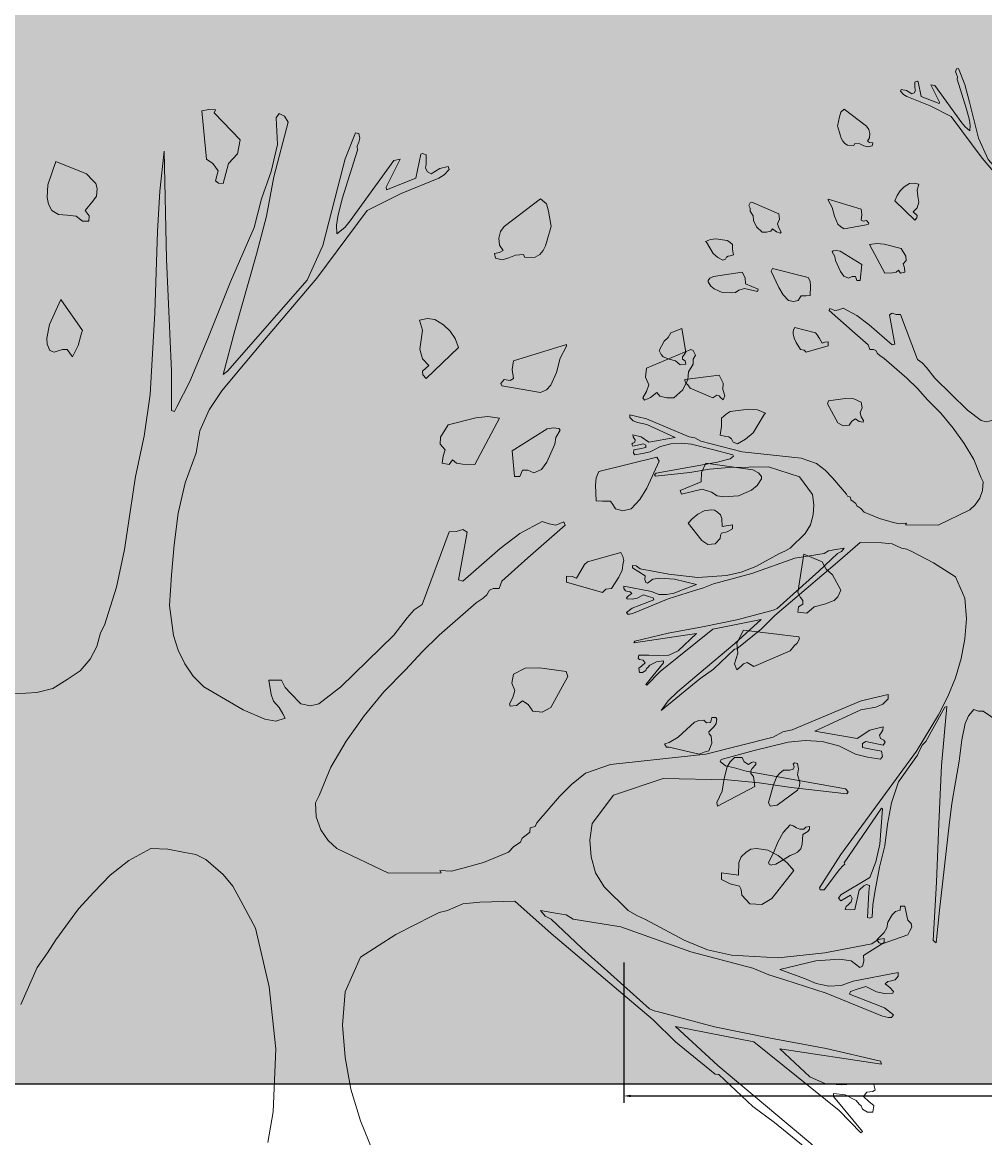
# Model space of a CAD drawing. Units: inches. Extents: x 84 to 1044, y -280 to 906.
# Tile 18 of 105: x 659 to 684, y -114 to -86. Entities that reach past the tile are written whole.
import ezdxf

# ---------------------------------------------------------------- set-up
doc = ezdxf.new("R2010")
doc.units = ezdxf.units.IN
for name, color, linetype, lineweight in [('A-ANNO-DIMS', 2, 'Continuous', 18), ('C-PROP', 7, 'Continuous', 25), ('L-PLNT', 114, 'Continuous', 15)]:
    doc.layers.add(name, color=color, linetype=linetype, lineweight=lineweight)
doc.layers.add('L-PLNT-PATT', color=9, linetype='Continuous', lineweight=9, true_color=0xafd9aa)
doc.styles.get("Standard").update_dxf_attribs({"font": 'arial.ttf'})
doc.dimstyles.get("Standard").update_dxf_attribs({"dimtxt": 0.18, "dimasz": 0.18, "dimexe": 0.18, "dimexo": 0.0625, "dimgap": 0.09, "dimtad": 0, "dimtih": 1, "dimtoh": 1, "dimdec": 4, "dimzin": 0, "dimdsep": 46, "dimtxsty": 'Standard', "dimcen": 0.09, "dimadec": 0, "dimazin": 0, "dimtfac": 1, "dimtdec": 4, "dimtofl": 0, "dimtmove": 0, "dimatfit": 3, "dimfxl": 1, "dimtolj": 1, "dimtzin": 0, "dimarcsym": 0})

# ---------------------------------------------------------------- blocks, each defined once
blk = doc.blocks.new('A$C37E508DF')
for p, q in [((0.6329, 1.5111), (0.6367, 1.5175)), ((0.6367, 1.5175), (0.6423, 1.5201)), ((0.6423, 1.5201), (0.6453, 1.5158)), ((0.6826, 1.493), (0.7096, 1.5209)), ((0.7083, 1.5239), (0.7152, 1.5244)), ((0.7096, 1.5209), (0.7083, 1.5239)), ((0.7152, 1.5244), (0.7225, 1.5231)), ((0.7225, 1.5231), (0.7174, 1.4729)), ((0.6475, 1.4545), (0.6329, 1.5111)), ((0.6453, 1.5158), (0.644, 1.4879)), ((0.5583, 1.4948), (0.5596, 1.4995)), ((0.5596, 1.4905), (0.5583, 1.4948)), ((0.5596, 1.4995), (0.563, 1.5003)), ((0.563, 1.5003), (0.5737, 1.4733)), ((0.6852, 1.4785), (0.6826, 1.493)), ((0.5613, 1.4862), (0.5596, 1.4905)), ((0.5608, 1.4823), (0.5613, 1.4862)), ((0.5767, 1.4317), (0.5608, 1.4823)), ((0.644, 1.4879), (0.6505, 1.46)), ((0.4897, 1.4772), (0.4935, 1.4789)), ((0.4897, 1.4678), (0.4897, 1.4772)), ((0.4935, 1.4789), (0.4952, 1.478)), ((0.4952, 1.478), (0.5004, 1.4532)), ((0.5313, 1.4437), (0.5167, 1.4729)), ((0.5167, 1.4729), (0.5231, 1.4716)), ((0.5231, 1.4716), (0.5686, 1.409)), ((0.5737, 1.4733), (0.5814, 1.4437)), ((0.6946, 1.4682), (0.6852, 1.4785)), ((0.7174, 1.4729), (0.7109, 1.4682)), ((0.7589, 1.3691), (0.7615, 1.481)), ((0.7615, 1.481), (0.7658, 1.4395)), ((0.8421, 1.4575), (0.8739, 1.4703)), ((0.8739, 1.4703), (0.882, 1.4463)), ((0.4657, 1.4622), (0.4669, 1.4652)), ((0.4708, 1.4566), (0.4657, 1.4622)), ((0.4669, 1.4652), (0.4755, 1.463)), ((0.4755, 1.463), (0.4845, 1.4575)), ((0.4845, 1.4575), (0.4884, 1.4596)), ((0.4884, 1.4596), (0.4905, 1.4635)), ((0.4905, 1.4635), (0.4897, 1.4678)), ((0.6505, 1.46), (0.6603, 1.4317)), ((0.6976, 1.4579), (0.6946, 1.4682)), ((0.7109, 1.4682), (0.7053, 1.4609)), ((0.7053, 1.4609), (0.7083, 1.4502)), ((0.4764, 1.4532), (0.4708, 1.4566)), ((0.5154, 1.4373), (0.4764, 1.4532)), ((0.5004, 1.4532), (0.5308, 1.4412)), ((0.6552, 1.4137), (0.6475, 1.4545)), ((0.7002, 1.4476), (0.6976, 1.4579)), ((0.7049, 1.448), (0.7002, 1.4476)), ((0.7083, 1.4502), (0.7049, 1.448)), ((0.831, 1.4424), (0.8323, 1.4476)), ((0.8323, 1.4476), (0.8357, 1.451)), ((0.8357, 1.451), (0.8421, 1.4575)), ((0.551, 1.4197), (0.5154, 1.4373)), ((0.5308, 1.4412), (0.5313, 1.4437)), ((0.5814, 1.4437), (0.5969, 1.3833)), ((0.7658, 1.4395), (0.7684, 1.3979)), ((0.8318, 1.4343), (0.831, 1.4424)), ((0.882, 1.4463), (0.8829, 1.433)), ((0.3628, 1.4189), (0.3649, 1.4266)), ((0.3649, 1.4266), (0.3709, 1.4317)), ((0.3709, 1.4317), (0.4086, 1.403)), ((0.5814, 1.4133), (0.5767, 1.4317)), ((0.6603, 1.4317), (0.668, 1.4021)), ((0.8353, 1.4292), (0.8318, 1.4343)), ((0.8434, 1.4197), (0.8353, 1.4292)), ((0.8816, 1.4262), (0.8781, 1.4197)), ((0.8829, 1.433), (0.8816, 1.4262)), ((0.3598, 1.403), (0.3628, 1.4189)), ((0.6029, 1.3494), (0.551, 1.4197)), ((0.5827, 1.4043), (0.5814, 1.4133)), ((0.6655, 1.3743), (0.6552, 1.4137)), ((0.8391, 1.4141), (0.8434, 1.4197)), ((0.8395, 1.4086), (0.8391, 1.4141)), ((0.8528, 1.4137), (0.846, 1.4086)), ((0.8619, 1.4146), (0.8528, 1.4137)), ((0.8709, 1.4154), (0.8619, 1.4146)), ((0.8781, 1.4197), (0.8709, 1.4154)), ((0.3602, 1.4021), (0.3598, 1.403)), ((0.364, 1.3888), (0.3602, 1.4021)), ((0.4086, 1.403), (0.4125, 1.3979)), ((0.5686, 1.409), (0.5741, 1.4021)), ((0.5741, 1.4021), (0.5823, 1.3953)), ((0.5823, 1.3953), (0.5827, 1.4043)), ((0.668, 1.4021), (0.6925, 1.3455)), ((0.846, 1.4086), (0.8395, 1.4086)), ((0.3657, 1.3828), (0.364, 1.3888)), ((0.4125, 1.3979), (0.4142, 1.391)), ((0.4142, 1.391), (0.4134, 1.3837)), ((0.7684, 1.3979), (0.771, 1.3134)), ((0.3683, 1.3781), (0.3657, 1.3828)), ((0.3718, 1.3738), (0.3683, 1.3781)), ((0.4134, 1.3837), (0.4099, 1.3781)), ((0.4099, 1.3781), (0.4134, 1.376)), ((0.5969, 1.3833), (0.6132, 1.3472)), ((0.3765, 1.3713), (0.3718, 1.3738)), ((0.3872, 1.3708), (0.3765, 1.3713)), ((0.3885, 1.3738), (0.3872, 1.3708)), ((0.3971, 1.3734), (0.3885, 1.3738)), ((0.4039, 1.3704), (0.3971, 1.3734)), ((0.4108, 1.3683), (0.4039, 1.3704)), ((0.4176, 1.37), (0.4108, 1.3683)), ((0.4134, 1.376), (0.4189, 1.3751)), ((0.4189, 1.3751), (0.4176, 1.37)), ((0.6882, 1.2949), (0.6655, 1.3743)), ((0.7538, 1.2529), (0.7589, 1.3691)), ((0.6595, 1.2829), (0.6029, 1.3494)), ((0.6132, 1.3472), (0.6959, 1.2529)), ((0.6925, 1.3455), (0.7161, 1.2868)), ((0.846, 1.2949), (0.8687, 1.3271)), ((0.8687, 1.3271), (0.8803, 1.3014)), ((0.771, 1.3134), (0.7761, 1.2285)), ((0.4648, 1.2945), (0.4717, 1.3009)), ((0.4717, 1.3009), (0.4807, 1.3065)), ((0.4807, 1.3065), (0.4884, 1.3074)), ((0.4884, 1.3074), (0.4965, 1.3057)), ((0.4965, 1.3057), (0.4935, 1.2954)), ((0.8803, 1.3014), (0.8833, 1.2872)), ((0.4562, 1.2774), (0.4597, 1.2868)), ((0.4597, 1.2868), (0.4648, 1.2945)), ((0.4935, 1.2954), (0.4948, 1.2855)), ((0.4948, 1.2855), (0.4961, 1.2756)), ((0.7002, 1.2495), (0.6882, 1.2949)), ((0.7161, 1.2868), (0.7349, 1.2422)), ((0.8473, 1.2924), (0.846, 1.2949)), ((0.8507, 1.2795), (0.8473, 1.2924)), ((0.8833, 1.2872), (0.8829, 1.2808)), ((0.2101, 1.2696), (0.2127, 1.2744)), ((0.2127, 1.2744), (0.2152, 1.2752)), ((0.2152, 1.2752), (0.2611, 1.2559)), ((0.3439, 1.2804), (0.3992, 1.2636)), ((0.3439, 1.2787), (0.3439, 1.2804)), ((0.3507, 1.2662), (0.3439, 1.2787)), ((0.4897, 1.2452), (0.4562, 1.2774)), ((0.4961, 1.2756), (0.4935, 1.2658)), ((0.6865, 1.2508), (0.6595, 1.2829)), ((0.8567, 1.2679), (0.8507, 1.2795)), ((0.8619, 1.2752), (0.8567, 1.2679)), ((0.867, 1.2752), (0.8619, 1.2752)), ((0.8713, 1.2739), (0.867, 1.2752)), ((0.8756, 1.2726), (0.8713, 1.2739)), ((0.8799, 1.2744), (0.8756, 1.2726)), ((0.8829, 1.2808), (0.8799, 1.2744)), ((0.2127, 1.2654), (0.2101, 1.2696)), ((0.2127, 1.2602), (0.2127, 1.2654)), ((0.3546, 1.2516), (0.3507, 1.2662)), ((0.3992, 1.2636), (0.4005, 1.2546)), ((0.4935, 1.2658), (0.4867, 1.2589)), ((0.2174, 1.2521), (0.2127, 1.2602)), ((0.2182, 1.2443), (0.2174, 1.2521)), ((0.2611, 1.2559), (0.262, 1.2465)), ((0.3602, 1.2383), (0.3546, 1.2516)), ((0.4005, 1.2546), (0.3992, 1.2452)), ((0.4867, 1.2589), (0.4935, 1.2529)), ((0.4935, 1.2529), (0.4931, 1.2491)), ((0.7015, 1.2323), (0.6865, 1.2508)), ((0.6959, 1.2529), (0.7002, 1.2495)), ((0.7538, 1.2122), (0.7538, 1.2529)), ((0.2234, 1.2336), (0.2182, 1.2443)), ((0.262, 1.2465), (0.2586, 1.2388)), ((0.2586, 1.2388), (0.2611, 1.2319)), ((0.3992, 1.2452), (0.4026, 1.2431)), ((0.4026, 1.2431), (0.4086, 1.2443)), ((0.4086, 1.2443), (0.4121, 1.2401)), ((0.4121, 1.2401), (0.4112, 1.2375)), ((0.4931, 1.2491), (0.4897, 1.2452)), ((0.7349, 1.2422), (0.7482, 1.216)), ((0.2328, 1.2251), (0.2234, 1.2336)), ((0.2504, 1.2306), (0.2474, 1.2268)), ((0.2568, 1.2255), (0.2504, 1.2306)), ((0.2611, 1.2319), (0.265, 1.2251)), ((0.3649, 1.2336), (0.3602, 1.2383)), ((0.3709, 1.2306), (0.3649, 1.2336)), ((0.4112, 1.2375), (0.3709, 1.2306)), ((0.7148, 1.2126), (0.7015, 1.2323)), ((0.7761, 1.2285), (0.7821, 1.1856)), ((0.2401, 1.2251), (0.2328, 1.2251)), ((0.2474, 1.2268), (0.2401, 1.2251)), ((0.2633, 1.2229), (0.2568, 1.2255)), ((0.265, 1.2251), (0.2633, 1.2229)), ((0.7482, 1.216), (0.7508, 1.2109)), ((0.1376, 1.2092), (0.1458, 1.2126)), ((0.1389, 1.2079), (0.1376, 1.2092)), ((0.1505, 1.189), (0.1389, 1.2079)), ((0.1458, 1.2126), (0.1548, 1.2135)), ((0.1548, 1.2135), (0.1741, 1.2109)), ((0.1741, 1.2109), (0.1784, 1.2083)), ((0.1784, 1.2083), (0.1831, 1.204)), ((0.1831, 1.204), (0.1831, 1.1959)), ((0.4134, 1.204), (0.4258, 1.2058)), ((0.4391, 1.156), (0.4134, 1.204)), ((0.4258, 1.2058), (0.4382, 1.2045)), ((0.4382, 1.2045), (0.4669, 1.1972)), ((0.7246, 1.1908), (0.7148, 1.2126)), ((0.7508, 1.2109), (0.7538, 1.2122)), ((0.1831, 1.1959), (0.1848, 1.1865)), ((0.3507, 1.1916), (0.352, 1.1933)), ((0.352, 1.1933), (0.3576, 1.1942)), ((0.3576, 1.1942), (0.364, 1.1929)), ((0.364, 1.1929), (0.4005, 1.1702)), ((0.4669, 1.1972), (0.4747, 1.1843)), ((0.1582, 1.1822), (0.1505, 1.189)), ((0.1668, 1.1775), (0.1582, 1.1822)), ((0.1728, 1.1826), (0.1711, 1.1792)), ((0.1758, 1.1847), (0.1728, 1.1826)), ((0.1788, 1.1852), (0.1758, 1.1847)), ((0.1848, 1.1865), (0.1788, 1.1852)), ((0.355, 1.1839), (0.3507, 1.1916)), ((0.3563, 1.177), (0.355, 1.1839)), ((0.4747, 1.1843), (0.4751, 1.177)), ((0.7281, 1.168), (0.7246, 1.1908)), ((0.7821, 1.1856), (0.7911, 1.1436)), ((0.1711, 1.1792), (0.1668, 1.1775)), ((0.3645, 1.1586), (0.3563, 1.177)), ((0.4005, 1.1702), (0.3979, 1.1436)), ((0.4751, 1.177), (0.47, 1.1714)), ((0.47, 1.1714), (0.4721, 1.1646)), ((0.2478, 1.1594), (0.2504, 1.1637)), ((0.2607, 1.1316), (0.2478, 1.1594)), ((0.2504, 1.1637), (0.3104, 1.1487)), ((0.37, 1.1509), (0.3645, 1.1586)), ((0.4622, 1.1607), (0.458, 1.1573)), ((0.4657, 1.156), (0.4622, 1.1607)), ((0.4721, 1.1646), (0.473, 1.1573)), ((0.7396, 1.1371), (0.7281, 1.168)), ((0.1419, 1.1436), (0.1449, 1.1474)), ((0.1449, 1.1474), (0.1509, 1.1504)), ((0.1509, 1.1504), (0.1994, 1.1573)), ((0.1994, 1.1573), (0.2041, 1.1479)), ((0.2041, 1.1479), (0.2045, 1.138)), ((0.3104, 1.1487), (0.3134, 1.1423)), ((0.3778, 1.1474), (0.37, 1.1509)), ((0.3842, 1.15), (0.3778, 1.1474)), ((0.3898, 1.15), (0.3842, 1.15)), ((0.3923, 1.1436), (0.3898, 1.15)), ((0.4519, 1.1564), (0.4391, 1.156)), ((0.458, 1.1573), (0.4519, 1.1564)), ((0.473, 1.1573), (0.4657, 1.156)), ((0.1419, 1.141), (0.1419, 1.1436)), ((0.1462, 1.1342), (0.1419, 1.141)), ((0.2045, 1.138), (0.226, 1.129)), ((0.3134, 1.1423), (0.3139, 1.1346)), ((0.3139, 1.1346), (0.3134, 1.1183)), ((0.3979, 1.1436), (0.3923, 1.1436)), ((0.7469, 1.1054), (0.7396, 1.1371)), ((0.7911, 1.1436), (0.8027, 1.0677)), ((0.1522, 1.1294), (0.1462, 1.1342)), ((0.1655, 1.1234), (0.1522, 1.1294)), ((0.181, 1.1226), (0.1655, 1.1234)), ((0.1878, 1.1234), (0.181, 1.1226)), ((0.1938, 1.1273), (0.1878, 1.1234)), ((0.2032, 1.1303), (0.1938, 1.1273)), ((0.2247, 1.1251), (0.2032, 1.1303)), ((0.226, 1.129), (0.2247, 1.1251)), ((0.268, 1.1196), (0.2607, 1.1316)), ((0.277, 1.1101), (0.268, 1.1196)), ((0.2959, 1.1144), (0.2933, 1.1101)), ((0.2984, 1.1179), (0.2959, 1.1144)), ((0.3066, 1.1179), (0.2984, 1.1179)), ((0.3134, 1.1183), (0.3066, 1.1179)), ((0.2856, 1.108), (0.277, 1.1101)), ((0.2933, 1.1101), (0.2856, 1.108)), ((0.7512, 1.0728), (0.7469, 1.1054)), ((0.3456, 1.093), (0.3469, 1.0964)), ((0.3842, 1.0591), (0.3456, 1.093)), ((0.3469, 1.0964), (0.355, 1.093)), ((0.355, 1.093), (0.3619, 1.0943)), ((0.3619, 1.0943), (0.3692, 1.0968)), ((0.3692, 1.0968), (0.3923, 1.0844)), ((0.4472, 1.0857), (0.4515, 1.0887)), ((0.4515, 1.0887), (0.4584, 1.0865)), ((0.3923, 1.0844), (0.4129, 1.069)), ((0.4562, 1.0364), (0.4472, 1.0857)), ((0.4584, 1.0865), (0.4657, 1.0861)), ((0.4657, 1.0861), (0.4939, 1.0107)), ((0.4129, 1.069), (0.4515, 1.0351)), ((0.7538, 1.0415), (0.7512, 1.0728)), ((0.8027, 1.0677), (0.8108, 1.0287)), ((0.0746, 1.0475), (0.0789, 1.0552)), ((0.0789, 1.0552), (0.0978, 1.063)), ((0.0978, 1.063), (0.1042, 1.0231)), ((0.2847, 1.0565), (0.2856, 1.0604)), ((0.2851, 1.054), (0.2847, 1.0565)), ((0.2864, 1.0463), (0.2851, 1.054)), ((0.2856, 1.0604), (0.2877, 1.0647)), ((0.2877, 1.0647), (0.3224, 1.0552)), ((0.3224, 1.0552), (0.3255, 1.0522)), ((0.4112, 1.0351), (0.3842, 1.0591)), ((0.0682, 1.0415), (0.0746, 1.0475)), ((0.2899, 1.039), (0.2864, 1.0463)), ((0.3255, 1.0522), (0.3293, 1.0458)), ((0.3293, 1.0458), (0.3336, 1.0381)), ((0.0596, 1.0257), (0.0682, 1.0415)), ((0.2972, 1.0274), (0.2899, 1.039)), ((0.3439, 1.0338), (0.3066, 1.0231)), ((0.3336, 1.0381), (0.3383, 1.0398)), ((0.3383, 1.0398), (0.3439, 1.0402)), ((0.3439, 1.0402), (0.3439, 1.0338)), ((0.4138, 1.0274), (0.4112, 1.0351)), ((0.4515, 1.0351), (0.4562, 1.0364)), ((0.7559, 1.0098), (0.7538, 1.0415)), ((0.0626, 1.0188), (0.0596, 1.0257)), ((0.0665, 1.0149), (0.0626, 1.0188)), ((0.1042, 1.0231), (0.1012, 1.018)), ((0.3032, 1.0265), (0.2972, 1.0274)), ((0.3066, 1.0231), (0.3032, 1.0265)), ((0.4202, 1.0274), (0.4138, 1.0274)), ((0.4241, 1.0257), (0.4202, 1.0274)), ((0.4267, 1.0209), (0.4241, 1.0257)), ((0.4305, 1.0175), (0.4267, 1.0209)), ((0.8108, 1.0287), (0.8233, 0.9892)), ((0.0763, 1.0111), (0.0665, 1.0149)), ((0.087, 1.0085), (0.0763, 1.0111)), ((0.0948, 1.0016), (0.087, 1.0085)), ((0.1012, 1.018), (0.099, 1.0149)), ((0.099, 1.0149), (0.099, 1.0111)), ((0.099, 1.0111), (0.1033, 1.0085)), ((0.1033, 1.0085), (0.1042, 1.0029)), ((0.4378, 1.0124), (0.4305, 1.0175)), ((0.476, 0.9789), (0.4378, 1.0124)), ((0.4939, 1.0107), (0.5021, 1.0051)), ((0.7516, 0.9785), (0.7559, 1.0098)), ((0.1042, 1.0029), (0.0948, 1.0016)), ((0.5021, 1.0051), (0.5094, 0.9969)), ((0.5094, 0.9969), (0.5231, 0.9789)), ((0.1029, 0.9772), (0.1604, 0.9841)), ((0.1604, 0.9841), (0.1672, 0.9708)), ((0.8233, 0.9892), (0.8275, 0.9815)), ((0.1025, 0.9751), (0.1029, 0.9772)), ((0.1046, 0.9708), (0.1025, 0.9751)), ((0.4939, 0.9618), (0.476, 0.9789)), ((0.5231, 0.9789), (0.578, 0.9253)), ((0.7469, 0.9635), (0.7516, 0.9785)), ((0.8275, 0.9815), (0.8314, 0.9673)), ((0.1076, 0.9682), (0.1046, 0.9708)), ((0.1119, 0.9626), (0.1076, 0.9682)), ((0.1496, 0.9463), (0.1119, 0.9626)), ((0.1672, 0.9708), (0.1664, 0.9601)), ((0.5111, 0.9429), (0.4939, 0.9618)), ((0.7401, 0.9493), (0.7469, 0.9635)), ((0.8314, 0.9673), (0.8383, 0.954)), ((0.1565, 0.9506), (0.1496, 0.9463)), ((0.1604, 0.9493), (0.1565, 0.9506)), ((0.1629, 0.9468), (0.1604, 0.9493)), ((0.1664, 0.9601), (0.1698, 0.9493)), ((0.1698, 0.9493), (0.1672, 0.9429)), ((0.7315, 0.9365), (0.7401, 0.9493)), ((0.8383, 0.954), (0.8486, 0.942)), ((0.1672, 0.9429), (0.1629, 0.9468)), ((0.3426, 0.936), (0.3443, 0.9412)), ((0.3443, 0.9412), (0.3722, 0.9451)), ((0.3722, 0.9451), (0.3868, 0.9446)), ((0.3868, 0.9446), (0.3992, 0.9386)), ((0.3992, 0.9386), (0.4009, 0.9292)), ((0.5334, 0.9202), (0.5111, 0.9429)), ((0.8486, 0.942), (0.8619, 0.933)), ((0.3602, 0.9039), (0.3426, 0.936)), ((0.4009, 0.9292), (0.3975, 0.9215)), ((0.6359, 0.9245), (0.6397, 0.9322)), ((0.6397, 0.9322), (0.653, 0.9322)), ((0.653, 0.9322), (0.6505, 0.9172)), ((0.7203, 0.9253), (0.7315, 0.9365)), ((0.8619, 0.933), (0.8769, 0.9236)), ((0.0103, 0.9129), (0.0103, 0.9172)), ((0.0103, 0.9172), (0.0382, 0.9107)), ((0.3975, 0.9215), (0.3996, 0.9142)), ((0.554, 0.8953), (0.5334, 0.9202)), ((0.578, 0.9253), (0.6011, 0.9077)), ((0.6196, 0.9077), (0.6303, 0.9189)), ((0.6303, 0.9189), (0.6359, 0.9245)), ((0.6505, 0.9172), (0.6479, 0.9103)), ((0.6796, 0.9013), (0.7203, 0.9253)), ((0.8769, 0.9236), (0.8936, 0.9193)), ((0.8936, 0.9193), (0.9279, 0.9172)), ((0.0159, 0.9073), (0.0103, 0.9129)), ((0.0232, 0.9043), (0.0159, 0.9073)), ((0.0386, 0.9013), (0.0232, 0.9043)), ((0.0382, 0.9107), (0.1098, 0.8807)), ((0.3692, 0.8992), (0.3602, 0.9039)), ((0.3838, 0.9069), (0.379, 0.9)), ((0.3898, 0.9107), (0.3838, 0.9069)), ((0.3958, 0.906), (0.3898, 0.9107)), ((0.4026, 0.9052), (0.3958, 0.906)), ((0.3996, 0.9142), (0.4031, 0.9077)), ((0.4031, 0.9077), (0.4026, 0.9052)), ((0.6011, 0.9077), (0.6097, 0.9056)), ((0.6097, 0.9056), (0.6196, 0.9077)), ((0.6423, 0.9039), (0.6384, 0.8974)), ((0.6479, 0.9103), (0.6423, 0.9039)), ((0.0866, 0.8794), (0.0386, 0.9013)), ((0.379, 0.9), (0.3692, 0.8992)), ((0.5728, 0.8691), (0.554, 0.8953)), ((0.6384, 0.8974), (0.6359, 0.8927)), ((0.6359, 0.8927), (0.6457, 0.8897)), ((0.6457, 0.8897), (0.6569, 0.8919)), ((0.6569, 0.8919), (0.6796, 0.9013)), ((0.0159, 0.8803), (0.0154, 0.8837)), ((0.0154, 0.8837), (0.0292, 0.8803)), ((0.0176, 0.8777), (0.0159, 0.8803)), ((0.0292, 0.8803), (0.0424, 0.8717)), ((0.1098, 0.8807), (0.1196, 0.8786)), ((0.0133, 0.8679), (0.015, 0.87)), ((0.015, 0.87), (0.0184, 0.8717)), ((0.0334, 0.8687), (0.0154, 0.8649)), ((0.0193, 0.8752), (0.0176, 0.8777)), ((0.0184, 0.8717), (0.0193, 0.8752)), ((0.0369, 0.8666), (0.0334, 0.8687)), ((0.0424, 0.8717), (0.0866, 0.8794)), ((0.0789, 0.8687), (0.0617, 0.864)), ((0.0965, 0.8696), (0.0789, 0.8687)), ((0.1141, 0.8679), (0.0965, 0.8696)), ((0.1196, 0.8786), (0.1295, 0.873)), ((0.1295, 0.873), (0.1994, 0.8554)), ((0.5887, 0.8421), (0.5728, 0.8691)), ((0.0154, 0.8649), (0.0133, 0.8679)), ((0.0163, 0.8529), (0.0171, 0.8584)), ((0.0171, 0.8584), (0.0266, 0.8602)), ((0.0266, 0.8602), (0.0369, 0.8623)), ((0.0369, 0.8623), (0.0369, 0.8666)), ((0.0617, 0.864), (0.0442, 0.8554)), ((0.1492, 0.8593), (0.1141, 0.8679)), ((0.1835, 0.8499), (0.1492, 0.8593)), ((0.0184, 0.8503), (0.0163, 0.8529)), ((0.0317, 0.8524), (0.0184, 0.8503)), ((0.0442, 0.8554), (0.0317, 0.8524)), ((0.1792, 0.8434), (0.1848, 0.8477)), ((0.1848, 0.8477), (0.1835, 0.8499)), ((0.1994, 0.8554), (0.2984, 0.8447)), ((0.0545, 0.8194), (0.1578, 0.8378)), ((0.1578, 0.8378), (0.1698, 0.8413)), ((0.1698, 0.8413), (0.1792, 0.8434)), ((0.2984, 0.8447), (0.3242, 0.8357)), ((0.3242, 0.8357), (0.3387, 0.8241)), ((0.6007, 0.8125), (0.5887, 0.8421)), ((0.1441, 0.8258), (0.1111, 0.8207)), ((0.1771, 0.8288), (0.1441, 0.8258)), ((0.2436, 0.8301), (0.1771, 0.8288)), ((0.2954, 0.813), (0.2436, 0.8301)), ((0.3387, 0.8241), (0.3512, 0.8117)), ((0.0519, 0.8164), (0.0545, 0.8194)), ((0.0532, 0.8143), (0.0519, 0.8164)), ((0.1111, 0.8207), (0.0532, 0.8143)), ((0.3173, 0.7834), (0.2954, 0.813)), ((0.3512, 0.8117), (0.3748, 0.7842)), ((0.6046, 0.8048), (0.6007, 0.8125)), ((0.6037, 0.7903), (0.6046, 0.8048)), ((0.599, 0.777), (0.6037, 0.7903)), ((0.3199, 0.7662), (0.3173, 0.7834)), ((0.3748, 0.7842), (0.3765, 0.7804)), ((0.3765, 0.7804), (0.3816, 0.7791)), ((0.3816, 0.7791), (0.382, 0.7744)), ((0.5913, 0.7658), (0.599, 0.777)), ((0.3186, 0.7491), (0.3199, 0.7662)), ((0.382, 0.7744), (0.3859, 0.7714)), ((0.3859, 0.7714), (0.3902, 0.7684)), ((0.3902, 0.7684), (0.3919, 0.7641)), ((0.3919, 0.7641), (0.3988, 0.7598)), ((0.5823, 0.7577), (0.5913, 0.7658)), ((0.1244, 0.7504), (0.1351, 0.7559)), ((0.1351, 0.7559), (0.1471, 0.7577)), ((0.1471, 0.7577), (0.1527, 0.7568)), ((0.1527, 0.7568), (0.1578, 0.7538)), ((0.1578, 0.7538), (0.1629, 0.7491)), ((0.3988, 0.7598), (0.4043, 0.7538)), ((0.4043, 0.7538), (0.4301, 0.7431)), ((0.5287, 0.7319), (0.5823, 0.7577)), ((0.7401, 0.7534), (0.7285, 0.7512)), ((0.7577, 0.7568), (0.7401, 0.7534)), ((0.7752, 0.7577), (0.7577, 0.7568)), ((0.798, 0.7452), (0.7752, 0.7577)), ((0.1081, 0.7349), (0.1153, 0.7427)), ((0.1153, 0.7427), (0.1244, 0.7504)), ((0.1629, 0.7491), (0.1651, 0.7431)), ((0.1651, 0.7431), (0.1655, 0.7298)), ((0.3139, 0.7324), (0.3186, 0.7491)), ((0.4301, 0.7431), (0.4515, 0.7371)), ((0.7182, 0.7461), (0.7002, 0.7307)), ((0.7285, 0.7512), (0.7182, 0.7461)), ((0.8173, 0.7298), (0.798, 0.7452)), ((0.1312, 0.7058), (0.1081, 0.7349)), ((0.1655, 0.7298), (0.1831, 0.7324)), ((0.1831, 0.7324), (0.1831, 0.7255)), ((0.3049, 0.7178), (0.3139, 0.7324)), ((0.4515, 0.7371), (0.4635, 0.7341)), ((0.4635, 0.7341), (0.4755, 0.7349)), ((0.4755, 0.7349), (0.4742, 0.7324)), ((0.4742, 0.7324), (0.5287, 0.7319)), ((0.7002, 0.7307), (0.6903, 0.7186)), ((0.8344, 0.7122), (0.8173, 0.7298)), ((0.1646, 0.7186), (0.1629, 0.7152)), ((0.1741, 0.7208), (0.1646, 0.7186)), ((0.1831, 0.7255), (0.1741, 0.7208)), ((0.28, 0.6933), (0.3049, 0.7178)), ((0.6903, 0.7186), (0.6818, 0.7032)), ((0.1621, 0.7092), (0.1539, 0.7002)), ((0.1629, 0.7152), (0.1621, 0.7092)), ((0.8503, 0.6951), (0.8344, 0.7122)), ((0.1415, 0.6994), (0.1312, 0.7058)), ((0.1539, 0.7002), (0.1415, 0.6994)), ((0.3975, 0.7028), (0.3598, 0.6693)), ((0.4339, 0.7019), (0.3975, 0.7028)), ((0.4515, 0.7002), (0.4339, 0.7019)), ((0.4674, 0.6933), (0.4515, 0.7002)), ((0.6818, 0.7032), (0.6667, 0.6749)), ((0.8739, 0.6629), (0.8503, 0.6951)), ((0.2221, 0.6625), (0.262, 0.6839)), ((0.262, 0.6839), (0.271, 0.6882)), ((0.271, 0.6882), (0.28, 0.6933)), ((0.337, 0.6843), (0.2877, 0.6762)), ((0.328, 0.6543), (0.3598, 0.6843)), ((0.3443, 0.6886), (0.337, 0.6843)), ((0.3533, 0.6903), (0.3443, 0.6886)), ((0.3709, 0.6933), (0.3533, 0.6903)), ((0.3598, 0.6843), (0.3662, 0.6873)), ((0.3662, 0.6873), (0.3709, 0.6933)), ((0.476, 0.6912), (0.4674, 0.6933)), ((0.4832, 0.6878), (0.476, 0.6912)), ((0.521, 0.6685), (0.4832, 0.6878)), ((0.2877, 0.6762), (0.2152, 0.6505)), ((0.6667, 0.6749), (0.6526, 0.614)), ((0.0146, 0.6599), (0.0146, 0.6642)), ((0.0146, 0.6642), (0.0206, 0.6633)), ((0.036, 0.6466), (0.0146, 0.6599)), ((0.0206, 0.6633), (0.0274, 0.6586)), ((0.1977, 0.6526), (0.2221, 0.6625)), ((0.3598, 0.6693), (0.2543, 0.5797)), ((0.5578, 0.6449), (0.521, 0.6685)), ((0.8824, 0.6492), (0.8739, 0.6629)), ((0.0274, 0.6586), (0.0759, 0.6492)), ((0.0759, 0.6492), (0.1244, 0.644)), ((0.2152, 0.6505), (0.1509, 0.6333)), ((0.1728, 0.647), (0.1977, 0.6526)), ((0.2581, 0.5913), (0.328, 0.6543)), ((0.8932, 0.6342), (0.8824, 0.6492)), ((0.0356, 0.6406), (0.036, 0.6466)), ((0.0369, 0.6355), (0.0356, 0.6406)), ((0.0489, 0.641), (0.0399, 0.6342)), ((0.0609, 0.6428), (0.0489, 0.641)), ((0.0853, 0.641), (0.0609, 0.6428)), ((0.1226, 0.632), (0.0853, 0.641)), ((0.1244, 0.644), (0.1728, 0.647)), ((0.5737, 0.6089), (0.5578, 0.6449)), ((0, 0.629), (0.0467, 0.62)), ((0, 0.6252), (0, 0.629)), ((0.003, 0.6213), (0, 0.6252)), ((0.0399, 0.6342), (0.0369, 0.6355)), ((0.0973, 0.6226), (0.1226, 0.632)), ((0.1342, 0.6265), (0.1175, 0.6213)), ((0.1509, 0.6333), (0.1342, 0.6265)), ((0.9103, 0.5956), (0.8932, 0.6342)), ((0.0069, 0.6204), (0.003, 0.6213)), ((0.0107, 0.6196), (0.0069, 0.6204)), ((0.0086, 0.6132), (0.0133, 0.617)), ((0.0133, 0.617), (0.0107, 0.6196)), ((0.0334, 0.6145), (0.0223, 0.6089)), ((0.0416, 0.6119), (0.0334, 0.6145)), ((0.0467, 0.62), (0.0592, 0.6153)), ((0.0592, 0.6153), (0.072, 0.6149)), ((0.072, 0.6149), (0.0849, 0.6175)), ((0.1175, 0.6213), (0.0746, 0.6076)), ((0.0849, 0.6175), (0.0973, 0.6226)), ((0.6526, 0.614), (0.6457, 0.5497)), ((0.0047, 0.6093), (0.0086, 0.6132)), ((0.0056, 0.6076), (0.0047, 0.6093)), ((0.0141, 0.6072), (0.0056, 0.6076)), ((0.0223, 0.6089), (0.0141, 0.6072)), ((0.0746, 0.6076), (0.0163, 0.5836)), ((0.0257, 0.5969), (0.0506, 0.6063)), ((0.0493, 0.6093), (0.0416, 0.6119)), ((0.0506, 0.6063), (0.0493, 0.6093)), ((0.5763, 0.5741), (0.5737, 0.6089)), ((0.0047, 0.5849), (0.0141, 0.5921)), ((0.0141, 0.5921), (0.0257, 0.5969)), ((0.253, 0.5892), (0.2581, 0.5913)), ((0.0069, 0.5823), (0.0047, 0.5849)), ((0.0099, 0.5823), (0.0069, 0.5823)), ((0.0163, 0.5836), (0.0099, 0.5823)), ((0.1904, 0.5724), (0.2474, 0.5879)), ((0.2543, 0.5797), (0.2311, 0.557)), ((0.2474, 0.5879), (0.253, 0.5892)), ((0.1325, 0.5608), (0.1904, 0.5724)), ((0.2311, 0.5729), (0.1496, 0.557)), ((0.1869, 0.5325), (0.2311, 0.5729)), ((0.5737, 0.5407), (0.5763, 0.5741)), ((0.1496, 0.557), (0.0613, 0.4858)), ((0.0746, 0.5501), (0.1325, 0.5608)), ((0.2311, 0.557), (0.1899, 0.5235)), ((0.1226, 0.5497), (0.0171, 0.5338)), ((0.0184, 0.5368), (0.0746, 0.5501)), ((0.0917, 0.5205), (0.1226, 0.5497)), ((0.6457, 0.5497), (0.6483, 0.4845)), ((0.0171, 0.5338), (0.0184, 0.5368)), ((0.1269, 0.482), (0.1869, 0.5325)), ((0.5677, 0.5077), (0.5737, 0.5407)), ((0.1861, 0.5231), (0.1509, 0.4897)), ((0.1899, 0.5235), (0.1861, 0.5231)), ((0.024, 0.5072), (0.0253, 0.5128)), ((0.0253, 0.5128), (0.042, 0.5133)), ((0.042, 0.5133), (0.0587, 0.5124)), ((0.0587, 0.5124), (0.0755, 0.5133)), ((0.0755, 0.5133), (0.0917, 0.5205)), ((0.0262, 0.5055), (0.024, 0.5072)), ((0.0326, 0.5047), (0.0262, 0.5055)), ((0.03, 0.4948), (0.036, 0.5004)), ((0.036, 0.5004), (0.0326, 0.5047)), ((0.0369, 0.4639), (0.0669, 0.5004)), ((0.0549, 0.5021), (0.0437, 0.4961)), ((0.0669, 0.5034), (0.0549, 0.5021)), ((0.0669, 0.5004), (0.0669, 0.5034)), ((0.5578, 0.4751), (0.5677, 0.5077)), ((0.0253, 0.491), (0.03, 0.4948)), ((0.0262, 0.4841), (0.0253, 0.491)), ((0.0369, 0.4871), (0.0317, 0.4841)), ((0.0382, 0.4905), (0.0369, 0.4871)), ((0.0403, 0.4922), (0.0382, 0.4905)), ((0.0437, 0.4961), (0.0403, 0.4922)), ((0.1509, 0.4897), (0.1282, 0.4734)), ((0.0317, 0.4841), (0.0262, 0.4841)), ((0.0613, 0.4858), (0.0386, 0.4627)), ((0.0905, 0.4515), (0.1269, 0.482)), ((0.545, 0.4434), (0.5578, 0.4751)), ((0.6483, 0.4845), (0.6539, 0.4524)), ((0.0386, 0.4627), (0.0369, 0.4639)), ((0.1282, 0.4734), (0.0626, 0.4198)), ((0.0746, 0.4361), (0.0905, 0.4515)), ((0.5295, 0.4125), (0.545, 0.4434)), ((0.0626, 0.4198), (0.0746, 0.4361)), ((0.5403, 0.4254), (0.5081, 0.3679)), ((0.5347, 0.3276), (0.5433, 0.4266)), ((0.5433, 0.4266), (0.5403, 0.4254)), ((0.5887, 0.4215), (0.5797, 0.4112)), ((0.5969, 0.4189), (0.5887, 0.4215)), ((0.6046, 0.4189), (0.5969, 0.4189)), ((0.6295, 0.4022), (0.6046, 0.4189)), ((0.1471, 0.4035), (0.1484, 0.4082)), ((0.1484, 0.4082), (0.1548, 0.4082)), ((0.1548, 0.4082), (0.1565, 0.4052)), ((0.1565, 0.4052), (0.1556, 0.3983)), ((0.4922, 0.3516), (0.5295, 0.4125)), ((0.5797, 0.4112), (0.5741, 0.3983)), ((0.1055, 0.388), (0.1192, 0.4001)), ((0.1192, 0.4001), (0.1265, 0.4031)), ((0.1265, 0.4031), (0.1346, 0.4039)), ((0.1346, 0.4039), (0.1389, 0.3992)), ((0.1389, 0.3992), (0.1458, 0.3996)), ((0.1458, 0.3996), (0.1471, 0.4035)), ((0.1556, 0.3983), (0.1518, 0.3932)), ((0.5741, 0.3983), (0.5686, 0.3705)), ((0.0917, 0.3748), (0.1055, 0.388)), ((0.1518, 0.3932), (0.1432, 0.3842)), ((0.1432, 0.3842), (0.1436, 0.3808)), ((0.0763, 0.3662), (0.0917, 0.3748)), ((0.1436, 0.3808), (0.1471, 0.3769)), ((0.1471, 0.3769), (0.1484, 0.3649)), ((0.5686, 0.3705), (0.5643, 0.3349)), ((0.069, 0.364), (0.0763, 0.3662)), ((0.069, 0.3627), (0.069, 0.364)), ((0.0716, 0.3585), (0.069, 0.3627)), ((0.1484, 0.3649), (0.1432, 0.352)), ((0.5025, 0.3619), (0.4982, 0.3537)), ((0.5081, 0.3679), (0.5025, 0.3619)), ((0.0763, 0.3585), (0.0716, 0.3585)), ((0.1269, 0.3464), (0.0763, 0.3585)), ((0.1355, 0.3499), (0.1269, 0.3464)), ((0.1432, 0.352), (0.1355, 0.3499)), ((0.4065, 0.2345), (0.4922, 0.3516)), ((0.4982, 0.3537), (0.4939, 0.3447)), ((0.1788, 0.3336), (0.1861, 0.3409)), ((0.1861, 0.3409), (0.199, 0.3409)), ((0.199, 0.3409), (0.2024, 0.3336)), ((0.4884, 0.337), (0.4622, 0.2997)), ((0.4939, 0.3447), (0.4884, 0.337)), ((0.1689, 0.3053), (0.1737, 0.325)), ((0.1737, 0.325), (0.1788, 0.3336)), ((0.2024, 0.3336), (0.2097, 0.3289)), ((0.2097, 0.3289), (0.2148, 0.3323)), ((0.2148, 0.3323), (0.2182, 0.3336)), ((0.2221, 0.3289), (0.2161, 0.3224)), ((0.2182, 0.3336), (0.2221, 0.3327)), ((0.2221, 0.3327), (0.2221, 0.3289)), ((0.2847, 0.3211), (0.2864, 0.325)), ((0.2851, 0.3302), (0.2877, 0.3319)), ((0.2864, 0.325), (0.2851, 0.3302)), ((0.2877, 0.3319), (0.292, 0.3306)), ((0.292, 0.3306), (0.2941, 0.322)), ((0.53, 0.229), (0.5347, 0.3276)), ((0.5643, 0.3349), (0.5578, 0.2993)), ((0.2161, 0.3224), (0.214, 0.3186)), ((0.214, 0.3186), (0.214, 0.3139)), ((0.214, 0.3139), (0.2182, 0.3087)), ((0.2577, 0.3087), (0.2624, 0.3147)), ((0.2624, 0.3147), (0.2689, 0.3194)), ((0.2689, 0.3194), (0.2796, 0.3194)), ((0.2796, 0.3194), (0.2847, 0.3211)), ((0.2941, 0.322), (0.292, 0.3117)), ((0.1655, 0.2843), (0.1689, 0.3053)), ((0.2182, 0.3087), (0.2204, 0.292)), ((0.2517, 0.2946), (0.2577, 0.3087)), ((0.292, 0.3117), (0.2959, 0.2993)), ((0.2204, 0.292), (0.1578, 0.259)), ((0.2436, 0.265), (0.2517, 0.2946)), ((0.2954, 0.2928), (0.292, 0.286)), ((0.2959, 0.2993), (0.2954, 0.2928)), ((0.4622, 0.2997), (0.4502, 0.2645)), ((0.5578, 0.2993), (0.5518, 0.2633)), ((0.1565, 0.265), (0.1655, 0.2843)), ((0.292, 0.286), (0.2581, 0.2607)), ((0.1578, 0.259), (0.1565, 0.265)), ((0.2461, 0.259), (0.2436, 0.265)), ((0.2581, 0.2607), (0.2461, 0.259)), ((0.4335, 0.2556), (0.3709, 0.1634)), ((0.4352, 0.2543), (0.4335, 0.2556)), ((0.4502, 0.2645), (0.4438, 0.2285)), ((0.5518, 0.2633), (0.5475, 0.2268)), ((0.4305, 0.1951), (0.4352, 0.2543)), ((0.3649, 0.1775), (0.4065, 0.2345)), ((0.268, 0.2148), (0.28, 0.2277)), ((0.28, 0.2277), (0.2851, 0.226)), ((0.2851, 0.226), (0.2903, 0.2225)), ((0.2903, 0.2225), (0.2963, 0.22)), ((0.2963, 0.22), (0.3027, 0.2204)), ((0.3027, 0.2204), (0.3061, 0.2234)), ((0.3061, 0.2234), (0.3122, 0.2247)), ((0.3122, 0.22), (0.3096, 0.2165)), ((0.3122, 0.2247), (0.3122, 0.22)), ((0.4438, 0.2285), (0.4391, 0.1921)), ((0.5261, 0.1308), (0.53, 0.229)), ((0.5475, 0.2268), (0.5313, 0.084)), ((0.2594, 0.1981), (0.268, 0.2148)), ((0.301, 0.211), (0.3002, 0.1951)), ((0.3096, 0.2165), (0.301, 0.211)), ((0.2521, 0.1805), (0.2594, 0.1981)), ((0.298, 0.1874), (0.292, 0.1818)), ((0.3002, 0.1951), (0.298, 0.1874)), ((0.4241, 0.1651), (0.4305, 0.1951)), ((0.4391, 0.1921), (0.4301, 0.1561)), ((0.2436, 0.1642), (0.2521, 0.1805)), ((0.28, 0.1762), (0.2684, 0.1689)), ((0.2873, 0.1788), (0.28, 0.1762)), ((0.292, 0.1818), (0.2873, 0.1788)), ((0.3293, 0.1213), (0.3649, 0.1775)), ((0.2448, 0.1616), (0.2436, 0.1642)), ((0.2684, 0.1689), (0.2556, 0.1616)), ((0.3709, 0.1634), (0.3718, 0.1616)), ((0.4138, 0.1389), (0.4241, 0.1651)), ((0.2478, 0.1599), (0.2448, 0.1616)), ((0.2508, 0.1608), (0.2478, 0.1599)), ((0.2556, 0.1616), (0.2508, 0.1608)), ((0.3628, 0.1526), (0.337, 0.1183)), ((0.3692, 0.1591), (0.3628, 0.1526)), ((0.3718, 0.1616), (0.3692, 0.1591)), ((0.4301, 0.1561), (0.4224, 0.1145)), ((0.3653, 0.1098), (0.4138, 0.1389)), ((0.5205, 0.033), (0.5261, 0.1308)), ((0.3306, 0.1183), (0.3293, 0.1213)), ((0.337, 0.1183), (0.3306, 0.1183)), ((0.3962, 0.1175), (0.3885, 0.0853)), ((0.4039, 0.1248), (0.3962, 0.1175)), ((0.4082, 0.1269), (0.4039, 0.1248)), ((0.4134, 0.1256), (0.4082, 0.1269)), ((0.4121, 0.1145), (0.4134, 0.1256)), ((0.3615, 0.1042), (0.3653, 0.1098)), ((0.3653, 0.0999), (0.3615, 0.1042)), ((0.3812, 0.1089), (0.3653, 0.0999)), ((0.3842, 0.1037), (0.3812, 0.1089)), ((0.4099, 0.0716), (0.4121, 0.1145)), ((0.4224, 0.1145), (0.4189, 0.093)), ((0.3739, 0.09), (0.3782, 0.0935)), ((0.3782, 0.0935), (0.3825, 0.0978)), ((0.3825, 0.0978), (0.3842, 0.1037)), ((0.4189, 0.093), (0.4176, 0.072)), ((0.3722, 0.0853), (0.3739, 0.09)), ((0.3808, 0.0845), (0.3722, 0.0853)), ((0.3885, 0.0853), (0.3808, 0.0845)), ((0.4515, 0.0763), (0.4571, 0.0815)), ((0.4571, 0.0815), (0.4648, 0.084)), ((0.4648, 0.084), (0.4657, 0.0905)), ((0.4657, 0.0905), (0.473, 0.0905)), ((0.473, 0.0905), (0.476, 0.0746)), ((0.5313, 0.084), (0.5257, 0.0291)), ((0.4142, 0.0707), (0.4099, 0.0716)), ((0.4176, 0.072), (0.4142, 0.0707)), ((0.4442, 0.0639), (0.4515, 0.0763)), ((0.476, 0.0746), (0.4777, 0.0673)), ((0.4425, 0.0544), (0.4442, 0.0639)), ((0.4777, 0.0673), (0.4832, 0.0613)), ((0.4832, 0.0613), (0.4845, 0.0553)), ((0.4378, 0.0463), (0.4425, 0.0544)), ((0.4811, 0.0493), (0.4777, 0.0424)), ((0.4845, 0.0553), (0.4811, 0.0493)), ((0.4258, 0.0339), (0.4378, 0.0463)), ((0.4777, 0.0424), (0.4348, 0.0274)), ((0.4296, 0.0291), (0.4258, 0.0339)), ((0.4348, 0.0274), (0.4296, 0.0291)), ((0.5257, 0.0291), (0.5205, 0.033))]:
    blk.add_line(p, q)
blk = doc.blocks.new('*D31')
at = {"layer": 'A-ANNO-DIMS', "color": 0, "lineweight": -2, "transparency": 16777216}
for p, q in [((674.751, -109.766), (674.751, -113.358)), ((696.24, -109.766), (696.24, -113.358)), ((674.931, -113.178), (684.966, -113.178)), ((696.06, -113.178), (686.025, -113.178))]:
    blk.add_line(p, q, dxfattribs=at)
at = {"layer": 'A-ANNO-DIMS', "color": 0, "transparency": 16777216}
for points in [[(674.931, -113.148), (674.931, -113.208), (674.751, -113.178)], [(696.06, -113.148), (696.06, -113.208), (696.24, -113.178)]]:
    blk.add_solid(points, dxfattribs=at)
at = {"layer": 'Defpoints', "color": 0, "transparency": 16777216}
for p in [(674.751, -109.703), (696.24, -109.703), (696.24, -113.178)]:
    blk.add_point(p, dxfattribs=at)
at = {"layer": 'A-ANNO-DIMS', "color": 0, "transparency": 16777216, "insert": (685.496, -113.178), "char_height": 0.18, "attachment_point": 5}
blk.add_mtext('\\A1;21 TYP.', dxfattribs=at)

msp = doc.modelspace()

# ---------------------------------------------------------------- hatches: boundary and pattern name
at = {"layer": 'L-PLNT-PATT', "transparency": 33554597}
h = msp.add_hatch(color=256, dxfattribs=at)
h.dxf.hatch_style = 1
h.paths.add_polyline_path([(791.074, 31.12), (791.074, 91.12), (743.074, 91.12), (674.074, 91.12), (674.074, 31.12), (650.074, 31.12), (650.074, -112.88), (983.074, -112.88), (983.074, -64.88), (791.074, -64.88)])

# ---------------------------------------------------------------- linework, layer by layer
at = {"layer": 'C-PROP'}
msp.add_lwpolyline([(143.179, -112.88), (143.179, 847.12), (983.074, 847.12), (983.074, -112.88), (624.574, -112.88)], dxfattribs=at)

# ---------------------------------------------------------------- block references
at = {"layer": 'L-PLNT'}
for p, xscale, yscale, zscale in [((674.751, -109.703, 0), 15.19586232982809, 15.19586232982809, 15.19586232982809), ((681.765, -125.52), -24.64361536662419, 24.64361536662419, 24.64361536662419)]:
    msp.add_blockref('A$C37E508DF', p, dxfattribs=dict(at, xscale=xscale, yscale=yscale, zscale=zscale))

# ---------------------------------------------------------------- dimensions: what is measured, and where the dimension line sits
at = {"layer": 'A-ANNO-DIMS'}
dim = msp.add_linear_dim(base=(696.24, -113.178), p1=(674.751, -109.703), p2=(696.24, -109.703), text='<> TYP.', dimstyle='Standard', override={"dimdec": 0, "dimlfac": 1, "dimrnd": 0, "dimzin": 0, "dimdsep": 46, "dimlunit": 2}, dxfattribs=at)
dim.commit()
dim.dimension.update_dxf_attribs({"geometry": '*D31', "text_midpoint": (685.496, -113.178)})

doc.saveas('drawing.dxf')
